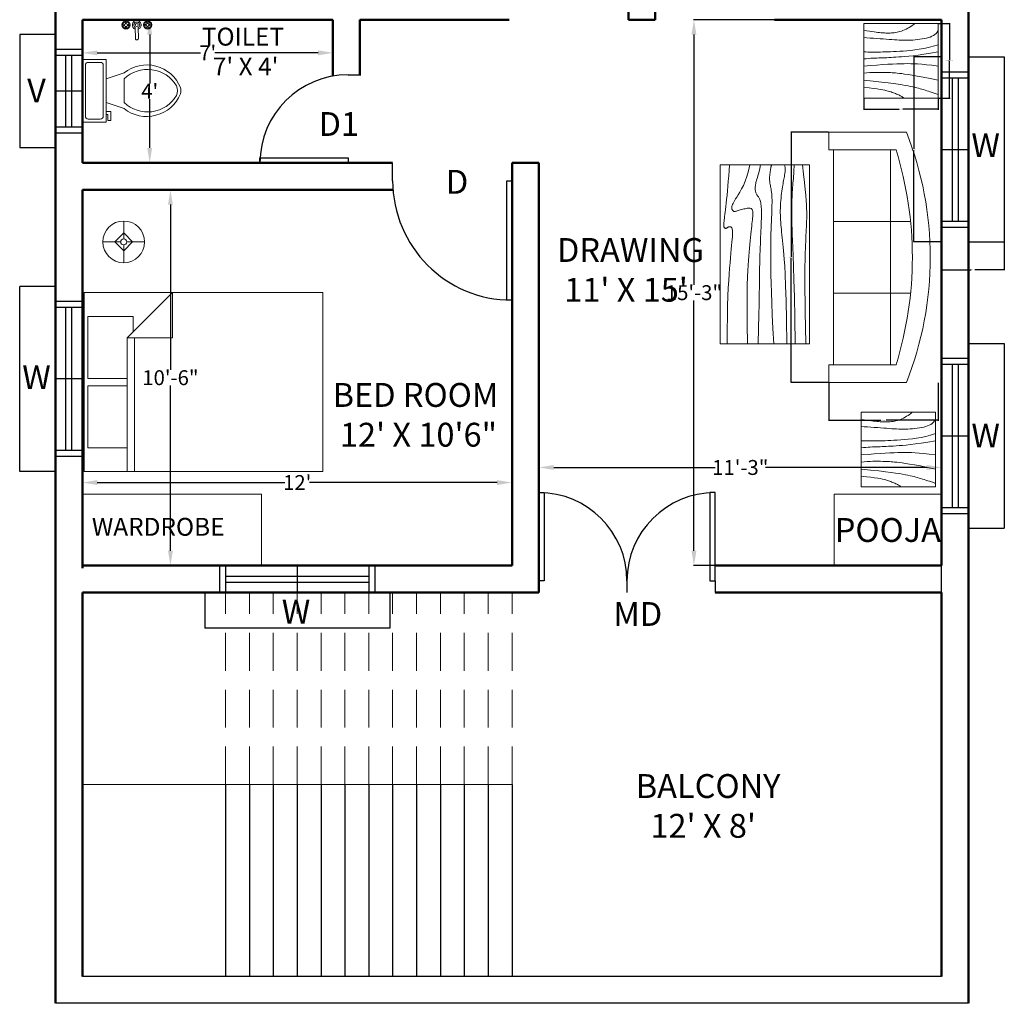
# Model space of a CAD drawing. Units: inches. Extents: x -25 to 789, y -921 to 230.
# Tile 4 of 5: x 437 to 767, y -323 to 6. Entities that reach past the tile are written whole.
import ezdxf

# ---------------------------------------------------------------- set-up
doc = ezdxf.new("R2010")
doc.units = ezdxf.units.IN
doc.header["$MEASUREMENT"] = 0
doc.linetypes.add('DASHED', pattern=[19.05, 12.7, -6.35])
for name, color, linetype, lineweight in [('A-ANNO-DIMS', 2, 'Continuous', 18), ('A-ANNO-TEXT', 7, 'Continuous', 18), ('A-AREA-IDEN', 3, 'Continuous', 18), ('A-DOOR', 4, 'Continuous', 25), ('A-ELEV', 7, 'Continuous', 25), ('A-FLOR-FIXT', 9, 'Continuous', 18), ('A-FLOR-OVHD', 8, 'DASHED', 18), ('A-FLOR-STRS', 3, 'Continuous', 25), ('A-FURN', 8, 'Continuous', 18), ('A-GLAZ', 4, 'Continuous', 25), ('A-WALL', 7, 'Continuous', 50), ('E-LITE-FIXT', 6, 'Continuous', 18)]:
    doc.layers.add(name, color=color, linetype=linetype, lineweight=lineweight)
doc.styles.get("Standard").update_dxf_attribs({"font": 'arial.ttf'})
doc.dimstyles.get("Standard").update_dxf_attribs({"dimtxt": 0.18, "dimasz": 0.18, "dimexe": 0.18, "dimexo": 0.0625, "dimgap": 0.09, "dimtad": 0, "dimtih": 1, "dimtoh": 1, "dimdec": 1, "dimzin": 0, "dimdsep": 46, "dimlunit": 4, "dimtxsty": 'Standard', "dimcen": 0.09, "dimadec": 0, "dimazin": 0, "dimtfac": 1, "dimtdec": 1, "dimtofl": 0, "dimtmove": 0, "dimatfit": 3, "dimfxl": 1, "dimtolj": 1, "dimtzin": 0, "dimarcsym": 0})

# ---------------------------------------------------------------- blocks, each defined once
blk = doc.blocks.new('Toilet - top')
for p, q in [((9.5, -6), (9.5, -2)), ((-10, -8.5), (-8, -8.5)), ((-10, -9.5), (-10, -8.5)), ((-7, -9.5), (-10, -9.5)), ((-8, -8.5), (-8, -8)), ((-7, -8), (-7, -9.5)), ((-4, -8), (-6, -14)), ((4, -8), (6, -14)), ((4, -14), (-4, -14))]:
    blk.add_line(p, q)
blk.add_lwpolyline([(10.5, -8), (10.5, 0), (-10.5, 0), (-10.5, -8)], close=True)
for points in [[(-9.5, -2), (-9.5, -6)], [(8.5, -1), (-8.5, -1)], [(-8.5, -7), (8.5, -7)]]:
    blk.add_lwpolyline(points)
for centre, radius, start, end in [((-8.62, -1.88), 0.884, 81.8699, 188.1301), ((8.62, -1.88), 0.884, 351.8699, 98.1301), ((-8.62, -6.12), 0.884, 171.8699, 278.1301), ((8.62, -6.12), 0.884, 261.8699, 8.1301), ((3.52, -21.58), 12.17, 141.4691, 247.9714), ((4.2, -21.82), 11.33, 136.3677, 238.9468), ((-3.52, -21.58), 12.17, 292.0284, 38.5307), ((-4.2, -21.82), 11.33, 301.053, 43.6321), ((0, -27.88), 4, 245.7318, 294.2682), ((0, -29), 4, 254.8605, 285.1395)]:
    blk.add_arc(centre, radius, start, end)
blk = doc.blocks.new('*U26')
for p, q in [((-40, 0), (-40, 6)), ((0, 0), (0, 6))]:
    blk.add_line(p, q)
blk.add_lwpolyline([(0, 0), (0, -40), (-1.75, -40), (-1.75, 0)], close=True)
blk.add_arc((0, 0), 40, 180, 270)
blk = doc.blocks.new('Faucet - Bathroom top')
for p, q in [((-4.107, 0.125), (-4.375, 0.125)), ((-3.75, 0.4788), (-3.75, 0.75)), ((-3.5, 0.482), (-3.5, 0.75)), ((-3.1461, 0.125), (-2.875, 0.125)), ((3.143, 0.125), (2.875, 0.125)), ((3.5, 0.4788), (3.5, 0.75)), ((3.75, 0.482), (3.75, 0.75)), ((4.1039, 0.125), (4.375, 0.125)), ((-4.1039, -0.125), (-4.375, -0.125)), ((-3.75, -0.4821), (-3.75, -0.75)), ((-3.5, -0.4789), (-3.5, -0.75)), ((-3.143, -0.125), (-2.875, -0.125)), ((-0.5, -0.8639), (-0.5, -4.5)), ((0.5, -4.5), (0.5, -0.8631)), ((3.1461, -0.125), (2.875, -0.125)), ((3.5, -0.4821), (3.5, -0.75)), ((3.75, -0.4789), (3.75, -0.75)), ((4.107, -0.125), (4.375, -0.125))]:
    blk.add_line(p, q)
for centre, radius in [((-3.625, 0), 1.375), ((-4.625, 0), 0.2795), ((-3.625, 0), 0.5), ((-3.625, 1), 0.2795), ((-2.625, 0), 0.2795), ((0, 0), 0.5), ((3.625, 0), 1.375), ((2.625, 0), 0.2795), ((3.625, 0), 0.5), ((3.625, 1), 0.2795), ((4.625, 0), 0.2795), ((-3.625, -1), 0.2795), ((3.625, -1), 0.2795)]:
    blk.add_circle(centre, radius)
for centre, radius, start, end in [((-3.625, 0), 1, 105.2407, 164.2093), ((-3.625, 0), 1, 16.44125, 74.07887), ((0, 0), 1.5, 289.6514, 250.3603), ((0, 0), 1, 300.3431, 239.7554), ((3.625, 0), 1, 106.12, 164.0884), ((3.625, 0), 1, 16.23422, 73.90469), ((-3.625, 0), 1, 196.2342, 253.9047), ((-3.625, 0), 1, 286.12, 344.0884), ((3.625, 0), 1, 196.4413, 254.0789), ((3.625, 0), 1, 285.2407, 344.2093), ((0, -4.5), 0.5, 180, 0)]:
    blk.add_arc(centre, radius, start, end)
blk = doc.blocks.new('*U20')
for p, q in [((-750, 0), (-750, 100)), ((0, 0), (0, 100))]:
    blk.add_line(p, q)
blk.add_lwpolyline([(0, 0), (0, -750), (-43.75, -750), (-43.75, 0)], close=True)
blk.add_arc((0, 0), 750, 180, 270)
blk = doc.blocks.new('Bed - Queen')
for p, q in [((0, -80.00003), (0, 0)), ((0, 0), (59.99999, 0)), ((59.99999, 0), (59.99999, -80.00003)), ((7.99999, -1.2), (28.79998, -1.2)), ((7.99999, -14.4), (7.99999, -1.2)), ((28.79998, -1.2), (28.79998, -14.4)), ((31.19999, -1.2), (51.99999, -1.2)), ((31.19999, -14.4), (31.19999, -1.2)), ((51.99999, -1.2), (51.99999, -16.4)), ((0, -14.4), (44.8, -14.4)), ((59.99999, -29.6), (44.8, -14.4)), ((44.8, -14.4), (44.8, -29.6)), ((51.99999, -16.4), (46.79936, -16.4)), ((44.8, -16.8), (0, -16.8)), ((44.8, -29.6), (59.99999, -29.6)), ((59.99999, -80.00003), (0, -80.00003))]:
    blk.add_line(p, q)
blk = doc.blocks.new('Lamp - Table')
for p, q in [((0, 7), (0, 1)), ((-1, 0), (-7, 0)), ((0, 3), (-3, 0)), ((-3, 0), (0, -3)), ((3, 0), (0, 3)), ((0, -3), (3, 0)), ((1, 0), (7, 0)), ((0, -1), (0, -7))]:
    blk.add_line(p, q)
for radius in [7, 1]:
    blk.add_circle((0, 0), radius)
blk = doc.blocks.new('*U4')
for p, q in [((-750, 0), (-750, -100)), ((0, 0), (0, -100))]:
    blk.add_line(p, q)
blk.add_lwpolyline([(0, 0), (0, 750), (-43.75, 750), (-43.75, 0)], close=True)
blk.add_arc((0, 0), 750, 90, 180)
blk = doc.blocks.new('*U11')
for p, q in [((0, 0), (0, -100)), ((750, 0), (750, -100))]:
    blk.add_line(p, q)
blk.add_lwpolyline([(0, 0), (0, 750), (43.75, 750), (43.75, 0)], close=True)
blk.add_arc((0, 0), 750, 0, 90)
blk = doc.blocks.new('Sofa - Roundback 7 ft.')
for p, q in [((-12.00002, -32.4421), (-12.00003, -6.5971)), ((11.99997, -32.4421), (11.99998, -6.5971)), ((-36.000027, -34), (-36.000027, -11.4696)), ((35.99998, -34), (35.99998, -11.4696)), ((-35.999844, -13.3819), (35.9998, -13.3819)), ((-36.000027, -32.4421), (35.99998, -32.4421))]:
    blk.add_line(p, q)
for points in [[(-36.000027, -34), (-42.000027, -34), (-42.000027, -8)], [(41.99998, -8), (41.99998, -34), (35.99998, -34)]]:
    blk.add_lwpolyline(points)
for centre, radius, start, end in [((0, -114.25), 114.25, 68.43141, 111.5686), ((-0.00001, -127.1968), 121.1968, 72.72033, 107.2797)]:
    blk.add_arc(centre, radius, start, end)
blk = doc.blocks.new('Table - Rectangular Woodgrain 60 x 30 in.')
for p, q in [((0, 0), (0, -30)), ((60, 0), (0, 0)), ((60, -30), (60, 0)), ((0, -30), (60, -30))]:
    blk.add_line(p, q)
for points in [[(0, -2.4), (4.8155, -2.418), (9.0302, -2.4688), (12.709, -2.5477), (15.9167, -2.65), (18.7181, -2.7711), (21.1781, -2.9063), (23.3616, -3.0508), (25.3333, -3.2), (27.1477, -3.3495), (28.8172, -3.4958), (30.3437, -3.636), (31.7291, -3.7667), (32.9756, -3.8849), (34.0849, -3.9875), (35.059, -4.0714), (35.9, -4.1334), (36.6114, -4.1711), (37.2041, -4.1854), (37.6906, -4.1779), (38.0833, -4.15), (38.3948, -4.1034), (38.6375, -4.0396), (38.8239, -3.9602), (38.9666, -3.8667), (39.0764, -3.7608), (39.1573, -3.6448), (39.2116, -3.521), (39.2416, -3.3917), (39.2498, -3.2593), (39.2385, -3.1261), (39.21, -2.9944), (39.1666, -2.8667), (39.111, -2.7447), (39.0468, -2.6281), (38.978, -2.5163), (38.9083, -2.4083), (38.8418, -2.3035), (38.7823, -2.201), (38.7337, -2.1001), (38.7, -2), (38.6844, -1.9003), (38.6875, -1.8021), (38.7094, -1.707), (38.75, -1.6167), (38.8094, -1.5326), (38.8875, -1.4563), (38.9844, -1.3893), (39.1, -1.3333), (39.2351, -1.2896), (39.3937, -1.2583), (39.5804, -1.2396), (39.8, -1.2333), (40.057, -1.2396), (40.3562, -1.2583), (40.7023, -1.2896), (41.1, -1.3333), (41.5547, -1.3895), (42.0755, -1.4573), (42.6721, -1.5361), (43.3542, -1.625), (44.1316, -1.7233), (45.014, -1.8302), (46.0114, -1.9449), (47.1333, -2.0667), (48.3862, -2.1947), (49.7625, -2.3281), (51.2513, -2.4663), (52.8416, -2.6083), (54.5226, -2.7535), (56.2833, -2.9011), (58.1127, -3.0501), (60, -3.2)], [(0, -9.2), (6.5759, -9.0858), (11.9385, -9.0365), (16.2527, -9.0418), (19.6833, -9.0917), (22.3952, -9.1759), (24.5531, -9.2844), (26.322, -9.4069), (27.8666, -9.5333), (29.3241, -9.6553), (30.7203, -9.7719), (32.0532, -9.8837), (33.3208, -9.9917), (34.5213, -10.0965), (35.6526, -10.199), (36.7128, -10.2999), (37.7, -10.4), (38.6129, -10.4996), (39.4531, -10.5969), (40.223, -10.6895), (40.925, -10.775), (41.5613, -10.8512), (42.1344, -10.9156), (42.6465, -10.966), (43.1, -11), (43.4976, -11.0158), (43.8437, -11.0136), (44.143, -10.9942), (44.4, -10.9583), (44.6195, -10.9069), (44.8062, -10.8406), (44.9648, -10.7603), (45.1, -10.6667), (45.2155, -10.5598), (45.3114, -10.4365), (45.3871, -10.2929), (45.4416, -10.125), (45.4743, -9.929), (45.4844, -9.7011), (45.4709, -9.4371), (45.4333, -9.1333), (45.3716, -8.7883), (45.2896, -8.4104), (45.1919, -8.0107), (45.0833, -7.6), (44.9685, -7.1893), (44.8521, -6.7896), (44.7388, -6.4117), (44.6333, -6.0667), (44.54, -5.7628), (44.4614, -5.4979), (44.4001, -5.2675), (44.3583, -5.0667), (44.3384, -4.8909), (44.3427, -4.7354), (44.3736, -4.5956), (44.4333, -4.4667), (44.5236, -4.3453), (44.6427, -4.2333), (44.7884, -4.1339), (44.9583, -4.05), (45.1501, -3.9849), (45.3614, -3.9417), (45.59, -3.9234), (45.8333, -3.9333), (46.0915, -3.9749), (46.3734, -4.0531), (46.6906, -4.1736), (47.0542, -4.3417), (47.4756, -4.5629), (47.9661, -4.8427), (48.5372, -5.1866), (49.2, -5.6), (49.9676, -6.0844), (50.8594, -6.625), (51.8965, -7.2031), (53.1, -7.8), (54.491, -8.3969), (56.0906, -8.975), (57.9199, -9.5156), (60, -10)], [(0, -12.8), (5.1847, -12.9322), (9.6213, -13.0323), (13.3963, -13.1059), (16.5958, -13.1583), (19.3063, -13.1952), (21.614, -13.2219), (23.6054, -13.2439), (25.3666, -13.2667), (26.9728, -13.2947), (28.4531, -13.3281), (29.8256, -13.3663), (31.1083, -13.4083), (32.3191, -13.4535), (33.476, -13.501), (34.597, -13.5501), (35.7, -13.6), (36.7984, -13.6497), (37.8875, -13.6979), (38.9578, -13.743), (40, -13.7833), (41.0047, -13.8174), (41.9625, -13.8438), (42.864, -13.8607), (43.7, -13.8667), (44.4631, -13.8604), (45.1552, -13.8417), (45.7801, -13.8104), (46.3416, -13.7667), (46.8439, -13.7104), (47.2906, -13.6417), (47.6858, -13.5604), (48.0333, -13.4667), (48.3375, -13.3608), (48.6042, -13.2448), (48.8396, -13.121), (49.05, -12.9917), (49.2417, -12.8593), (49.4208, -12.7261), (49.5937, -12.5944), (49.7667, -12.4667), (49.9452, -12.3451), (50.1323, -12.2313), (50.3303, -12.1268), (50.5416, -12.0333), (50.7686, -11.9524), (51.0135, -11.8854), (51.2788, -11.8341), (51.5666, -11.8), (51.8785, -11.7843), (52.2116, -11.7865), (52.562, -11.8059), (52.926, -11.8417), (53.2998, -11.8931), (53.6795, -11.9594), (54.0614, -12.0397), (54.4416, -12.1333), (54.8223, -12.2401), (55.2293, -12.3625), (55.6942, -12.5037), (56.2489, -12.6667), (56.9251, -12.8547), (57.7545, -13.0708), (58.7689, -13.3182), (60, -13.6)], [(0, -18), (5.124, -17.7273), (9.6609, -17.5057), (13.6705, -17.3303), (17.2125, -17.1958), (20.3467, -17.0973), (23.1328, -17.0297), (25.6307, -16.9878), (27.9, -16.9667), (29.9928, -16.9617), (31.9302, -16.9703), (33.7254, -16.9907), (35.3917, -17.0208), (36.9423, -17.0588), (38.3906, -17.1026), (39.7499, -17.1503), (41.0333, -17.2), (42.2519, -17.2496), (43.4073, -17.2969), (44.4986, -17.3395), (45.525, -17.375), (46.4858, -17.4012), (47.3802, -17.4156), (48.2074, -17.416), (48.9667, -17.4), (49.6583, -17.3662), (50.2872, -17.3167), (50.8595, -17.2547), (51.3812, -17.1833), (51.8584, -17.1057), (52.2971, -17.025), (52.7034, -16.9443), (53.0833, -16.8667), (53.443, -16.7951), (53.789, -16.7313), (54.128, -16.6768), (54.4666, -16.6334), (54.8115, -16.6024), (55.1693, -16.5854), (55.5465, -16.5841), (55.95, -16.6), (56.3828, -16.6337), (56.8346, -16.6823), (57.2915, -16.7418), (57.7396, -16.8084), (58.165, -16.878), (58.5539, -16.9469), (58.8924, -17.0111), (59.1666, -17.0667), (59.3679, -17.1107), (59.5078, -17.1438), (59.6032, -17.1675), (59.6708, -17.1833), (59.7275, -17.193), (59.7901, -17.1979), (59.8753, -17.1998), (60, -17.2)], [(0, -22.4), (8.0098, -22.2501), (14.4094, -22.1011), (19.4168, -21.9535), (23.25, -21.8083), (26.1269, -21.6663), (28.2656, -21.5281), (29.884, -21.3947), (31.2, -21.2667), (32.3967, -21.1448), (33.5172, -21.0292), (34.5697, -20.9198), (35.5625, -20.8167), (36.5037, -20.7198), (37.4015, -20.6292), (38.2642, -20.5448), (39.1, -20.4667), (39.9164, -20.3951), (40.7187, -20.3313), (41.5117, -20.2768), (42.3, -20.2333), (43.0883, -20.2024), (43.8812, -20.1854), (44.6836, -20.1841), (45.5, -20.2), (46.3328, -20.234), (47.1747, -20.2844), (48.0163, -20.3488), (48.8479, -20.425), (49.66, -20.5106), (50.4429, -20.6031), (51.1872, -20.7004), (51.8833, -20.8), (52.5246, -20.8999), (53.1166, -20.9995), (53.6681, -21.0983), (54.1875, -21.1958), (54.6834, -21.2919), (55.1646, -21.3859), (55.6394, -21.4777), (56.1167, -21.5667), (56.6028, -21.6515), (57.0961, -21.7266), (57.5929, -21.7852), (58.0896, -21.8208), (58.5823, -21.8268), (59.0674, -21.7964), (59.5412, -21.723), (60, -21.6)], [(0, -25.2), (8.6355, -25.0504), (15.7026, -24.9031), (21.4049, -24.7606), (25.9458, -24.625), (29.529, -24.4988), (32.3578, -24.3844), (34.6359, -24.284), (36.5667, -24.2), (38.3213, -24.1341), (39.9417, -24.0854), (41.437, -24.0523), (42.8167, -24.0333), (44.0901, -24.0268), (45.2667, -24.0313), (46.3557, -24.0451), (47.3667, -24.0667), (48.309, -24.0947), (49.1928, -24.1287), (50.0284, -24.168), (50.826, -24.2125), (51.5959, -24.2617), (52.3483, -24.3151), (53.0935, -24.3725), (53.8417, -24.4334), (54.6009, -24.497), (55.3699, -24.561), (56.1454, -24.6226), (56.9239, -24.6792), (57.7021, -24.7279), (58.4764, -24.7662), (59.2435, -24.7911), (60, -24.8)], [(0, -28.8), (5.6867, -28.6681), (10.45, -28.5698), (14.407, -28.5012), (17.675, -28.4584), (20.3711, -28.4374), (22.6125, -28.4344), (24.5164, -28.4455), (26.2, -28.4667), (27.762, -28.4947), (29.2276, -28.5281), (30.6033, -28.5663), (31.8958, -28.6084), (33.1118, -28.6535), (34.2578, -28.7011), (35.3405, -28.7501), (36.3666, -28.8), (37.3443, -28.8497), (38.288, -28.8974), (39.2137, -28.9412), (40.1375, -28.9792), (41.0753, -29.0093), (42.0432, -29.0297), (43.0572, -29.0384), (44.1333, -29.0333), (45.2936, -29.0114), (46.5843, -28.9641), (48.0579, -28.8816), (49.7666, -28.7542), (51.7629, -28.5721), (54.0989, -28.3255), (56.8272, -28.0048), (60, -27.6)]]:
    blk.add_lwpolyline(points)
blk = doc.blocks.new('Table - Square Woodgrain 42 x 42 in.')
blk.add_line((0, -42), (42, -42))
for points in [[(0, -4), (1.704, -4.2172), (3.2358, -4.4188), (4.615, -4.604), (5.8615, -4.7721), (6.9951, -4.9224), (8.0357, -5.0541), (9.0031, -5.1667), (9.9171, -5.2594), (10.7951, -5.3316), (11.6445, -5.3836), (12.4702, -5.4157), (13.277, -5.4283), (14.0698, -5.4217), (14.8535, -5.3964), (15.6331, -5.3526), (16.4133, -5.2908), (17.1986, -5.2103), (17.9913, -5.1062), (18.793, -4.9727), (19.6056, -4.8038), (20.4307, -4.5937), (21.2701, -4.3365), (22.1256, -4.0262), (22.9989, -3.6571), (23.888, -3.2272), (24.7756, -2.7516), (25.6408, -2.2491), (26.4624, -1.7387), (27.2195, -1.2395), (27.891, -0.7703), (28.456, -0.3501), (28.8934, 0.002)], [(0, -42), (0, 0), (42, 0), (42, -42)], [(0, -8), (1.8203, -8.1001), (3.6741, -8.2149), (5.5411, -8.3408), (7.4011, -8.4741), (9.2339, -8.6112), (11.0193, -8.7484), (12.7371, -8.8821), (14.3671, -9.0086), (15.8954, -9.1246), (17.3337, -9.2278), (18.6997, -9.3159), (20.0116, -9.387), (21.2871, -9.4389), (22.5442, -9.4696), (23.8008, -9.477), (25.0749, -9.459), (26.3791, -9.4137), (27.7049, -9.3403), (29.0383, -9.2382), (30.3655, -9.1068), (31.6728, -8.9455), (32.9461, -8.7535), (34.1717, -8.5304), (35.3358, -8.2756), (36.4268, -7.9863), (37.443, -7.6521), (38.3849, -7.2603), (39.253, -6.7986), (40.048, -6.2542), (40.7705, -5.6147), (41.421, -4.8674), (42, -4)], [(42, -12), (39.1784, -12.8621), (36.4519, -13.5654), (33.8246, -14.1294), (31.3004, -14.5731), (28.8832, -14.9161), (26.577, -15.1775), (24.3858, -15.3768), (22.3136, -15.5332), (20.3622, -15.6632), (18.5254, -15.7718), (16.7947, -15.8612), (15.1618, -15.9338), (13.6183, -15.9916), (12.1558, -16.0369), (10.7659, -16.0718), (9.4403, -16.0987), (8.1703, -16.1191), (6.9461, -16.1325), (5.7577, -16.1377), (4.595, -16.1335), (3.4479, -16.1188), (2.3064, -16.0924), (1.1604, -16.0532), (0, -16)], [(42, -16), (37.6529, -16.7365), (33.8802, -17.329), (30.6179, -17.7961), (27.8015, -18.1561), (25.3668, -18.4275), (23.2497, -18.6288), (21.3859, -18.7785), (19.7111, -18.8949), (18.1693, -18.9939), (16.7375, -19.0795), (15.401, -19.1534), (14.1449, -19.217), (12.9544, -19.2717), (11.8148, -19.3191), (10.7113, -19.3606), (9.6291, -19.3976), (8.5534, -19.4323), (7.47, -19.4689), (6.3643, -19.5122), (5.222, -19.5672), (4.0288, -19.6386), (2.7703, -19.7313), (1.4321, -19.8501), (0, -20)], [(0, -24), (3.9243, -23.6805), (7.4766, -23.4138), (10.6891, -23.1954), (13.5943, -23.0205), (16.2247, -22.8847), (18.6125, -22.7832), (20.7903, -22.7116), (22.7903, -22.6651), (24.6563, -22.642), (26.4764, -22.6507), (28.35, -22.7024), (30.3766, -22.8084), (32.6555, -22.98), (35.2861, -23.2283), (38.3678, -23.5645), (42, -24)], [(42, -32), (37.392, -31.017), (33.4585, -30.2231), (30.1291, -29.5949), (27.3334, -29.109), (25.0009, -28.742), (23.0612, -28.4707), (21.4439, -28.2716), (20.0786, -28.1215), (18.8998, -28.0002), (17.8609, -27.9014), (16.9206, -27.8219), (16.0371, -27.7588), (15.1691, -27.709), (14.2748, -27.6693), (13.3128, -27.6368), (12.2415, -27.6083), (11.0295, -27.5824), (9.6867, -27.5643), (8.233, -27.5608), (6.6884, -27.5787), (5.0728, -27.6248), (3.4062, -27.7058), (1.7086, -27.8286), (0, -28)], [(0, -32), (5.4026, -32.5358), (9.9494, -33.019), (13.7424, -33.4553), (16.8834, -33.8505), (19.4743, -34.2106), (21.6171, -34.5413), (23.4136, -34.8486), (24.9657, -35.1382), (26.3614, -35.4156), (27.6332, -35.6841), (28.7995, -35.9467), (29.8788, -36.2064), (30.8897, -36.4661), (31.8507, -36.7288), (32.7802, -36.9973), (33.6968, -37.2747), (34.6175, -37.5635), (35.5531, -37.8651), (36.5128, -38.1805), (37.506, -38.5108), (38.5421, -38.8568), (39.6302, -39.2197), (40.7797, -39.6004), (42, -40)], [(0, -36), (3.0098, -36.2857), (5.5354, -36.5643), (7.6368, -36.8359), (9.374, -37.1009), (10.807, -37.3597), (11.9957, -37.6126), (13.0002, -37.8599), (13.8804, -38.102), (14.6874, -38.3393), (15.4365, -38.5729), (16.1338, -38.8041), (16.7858, -39.0341), (17.3987, -39.264), (17.9787, -39.4952), (18.5322, -39.7288), (19.0655, -39.9662), (19.5832, -40.2081), (20.0842, -40.4544), (20.5657, -40.7046), (21.0249, -40.9581), (21.459, -41.2144), (21.8653, -41.4731), (22.2409, -41.7335), (22.5831, -41.9951)]]:
    blk.add_lwpolyline(points)
blk = doc.blocks.new('*D59')
at = {"layer": 'A-ANNO-DIMS', "color": 0, "lineweight": -2, "transparency": 16777216}
for p, q in [((458.24, -176.64), (458.24, -148.68)), ((463.24, -148.86), (526.14, -148.86)), ((597.24, -148.86), (534.33, -148.86)), ((602.24, -176.64), (602.24, -148.68))]:
    blk.add_line(p, q, dxfattribs=at)
at = {"layer": 'A-ANNO-DIMS', "color": 0, "transparency": 16777216}
for points in [[(463.24, -148.02), (463.24, -149.69), (458.24, -148.86)], [(597.24, -148.02), (597.24, -149.69), (602.24, -148.86)]]:
    blk.add_solid(points, dxfattribs=at)
at = {"layer": 'Defpoints', "color": 0, "transparency": 16777216}
for p in [(602.24, -148.86), (458.24, -176.7), (602.24, -176.7)]:
    blk.add_point(p, dxfattribs=at)
at = {"layer": 'A-ANNO-DIMS', "color": 0, "transparency": 16777216, "insert": (530.24, -148.86), "char_height": 5, "attachment_point": 5}
blk.add_mtext("\\A1;12'", dxfattribs=at)
blk = doc.blocks.new('*D60')
at = {"layer": 'A-ANNO-DIMS', "color": 0, "lineweight": -2, "transparency": 16777216}
for p, q in [((458.3, -50.7), (487.93, -50.7)), ((487.75, -55.7), (487.75, -111.06)), ((487.75, -171.7), (487.75, -116.35)), ((458.3, -176.7), (487.93, -176.7))]:
    blk.add_line(p, q, dxfattribs=at)
at = {"layer": 'A-ANNO-DIMS', "color": 0, "transparency": 16777216}
for points in [[(486.92, -55.7), (488.59, -55.7), (487.75, -50.7)], [(486.92, -171.7), (488.59, -171.7), (487.75, -176.7)]]:
    blk.add_solid(points, dxfattribs=at)
at = {"layer": 'Defpoints', "color": 0, "transparency": 16777216}
for p in [(458.24, -50.7), (487.75, -50.7), (458.24, -176.7)]:
    blk.add_point(p, dxfattribs=at)
at = {"layer": 'A-ANNO-DIMS', "color": 0, "transparency": 16777216, "insert": (487.75, -113.7), "char_height": 5, "attachment_point": 5}
blk.add_mtext('\\A1;10\'-6"', dxfattribs=at)
blk = doc.blocks.new('*D61')
at = {"layer": 'A-ANNO-DIMS', "color": 0, "lineweight": -2, "transparency": 16777216}
for p, q in [((458.3, 6.3), (480.99, 6.3)), ((480.81, 1.3), (480.81, -15.11)), ((480.81, -36.7), (480.81, -20.29)), ((458.3, -41.7), (480.99, -41.7))]:
    blk.add_line(p, q, dxfattribs=at)
at = {"layer": 'A-ANNO-DIMS', "color": 0, "transparency": 16777216}
for points in [[(479.97, 1.3), (481.64, 1.3), (480.81, 6.3)], [(479.97, -36.7), (481.64, -36.7), (480.81, -41.7)]]:
    blk.add_solid(points, dxfattribs=at)
at = {"layer": 'Defpoints', "color": 0, "transparency": 16777216}
for p in [(458.24, 6.3), (480.81, 6.3), (458.24, -41.7)]:
    blk.add_point(p, dxfattribs=at)
at = {"layer": 'A-ANNO-DIMS', "color": 0, "transparency": 16777216, "insert": (480.81, -17.7), "char_height": 5, "attachment_point": 5}
blk.add_mtext("\\A1;4'", dxfattribs=at)
blk = doc.blocks.new('*D62')
at = {"layer": 'A-ANNO-DIMS', "color": 0, "lineweight": -2, "transparency": 16777216}
for p, q in [((458.24, 6.23), (458.24, -5)), ((542.24, 6.23), (542.24, -5)), ((463.24, -4.82), (497.87, -4.82)), ((537.24, -4.82), (502.61, -4.82))]:
    blk.add_line(p, q, dxfattribs=at)
at = {"layer": 'A-ANNO-DIMS', "color": 0, "transparency": 16777216}
for points in [[(463.24, -3.99), (463.24, -5.65), (458.24, -4.82)], [(537.24, -3.99), (537.24, -5.65), (542.24, -4.82)]]:
    blk.add_solid(points, dxfattribs=at)
at = {"layer": 'Defpoints', "color": 0, "transparency": 16777216}
for p in [(458.24, 6.3), (542.24, 6.3), (542.24, -4.82)]:
    blk.add_point(p, dxfattribs=at)
at = {"layer": 'A-ANNO-DIMS', "color": 0, "transparency": 16777216, "insert": (500.24, -4.82), "char_height": 5, "attachment_point": 5}
blk.add_mtext("\\A1;7'", dxfattribs=at)
blk = doc.blocks.new('*D71')
at = {"layer": 'A-ANNO-DIMS', "color": 0, "lineweight": -2, "transparency": 16777216}
for p, q in [((611.24, -185.64), (611.24, -143.62)), ((616.24, -143.8), (670.29, -143.8)), ((741.24, -143.8), (687.18, -143.8)), ((746.24, -185.64), (746.24, -143.62))]:
    blk.add_line(p, q, dxfattribs=at)
at = {"layer": 'A-ANNO-DIMS', "color": 0, "transparency": 16777216}
for points in [[(616.24, -142.97), (616.24, -144.64), (611.24, -143.8)], [(741.24, -142.97), (741.24, -144.64), (746.24, -143.8)]]:
    blk.add_solid(points, dxfattribs=at)
at = {"layer": 'Defpoints', "color": 0, "transparency": 16777216}
for p in [(746.24, -143.8), (611.24, -185.7), (746.24, -185.7)]:
    blk.add_point(p, dxfattribs=at)
at = {"layer": 'A-ANNO-DIMS', "color": 0, "transparency": 16777216, "insert": (678.74, -143.8), "char_height": 5, "attachment_point": 5}
blk.add_mtext('\\A1;11\'-3"', dxfattribs=at)
blk = doc.blocks.new('*D72')
at = {"layer": 'A-ANNO-DIMS', "color": 0, "lineweight": -2, "transparency": 16777216}
for p, q in [((690.17, 6.3), (663.04, 6.3)), ((663.22, 1.3), (663.22, -82.56)), ((663.22, -171.7), (663.22, -87.85)), ((670.23, -176.7), (663.04, -176.7))]:
    blk.add_line(p, q, dxfattribs=at)
at = {"layer": 'A-ANNO-DIMS', "color": 0, "transparency": 16777216}
for points in [[(662.38, 1.3), (664.05, 1.3), (663.22, 6.3)], [(662.38, -171.7), (664.05, -171.7), (663.22, -176.7)]]:
    blk.add_solid(points, dxfattribs=at)
at = {"layer": 'Defpoints', "color": 0, "transparency": 16777216}
for p in [(663.22, 6.3), (690.24, 6.3), (670.29, -176.7)]:
    blk.add_point(p, dxfattribs=at)
at = {"layer": 'A-ANNO-DIMS', "color": 0, "transparency": 16777216, "insert": (663.22, -85.2), "char_height": 5, "attachment_point": 5}
blk.add_mtext('\\A1;15\'-3"', dxfattribs=at)
blk = doc.blocks.new('WIN-W-SUNSHADE')
at = {"ltscale": 2}
for p, q in [((0, 9), (0, 21)), ((0, 21), (62, 21)), ((62, 9), (62, 21)), ((5, 9), (0, 9)), ((57, 9), (62, 9))]:
    blk.add_line(p, q, dxfattribs=at)
for p, q in [((5, 0), (5, 9)), ((57, 0), (57, 9))]:
    blk.add_line(p, q)
blk = doc.blocks.new('WIN-V-SUNSHADE')
for p, q in [((0, 9), (0, 21)), ((38, 21), (0, 21)), ((38, 9), (38, 21)), ((5, 9), (0, 9)), ((5, 0), (5, 9)), ((33, 0), (33, 9)), ((33, 9), (38, 9))]:
    blk.add_line(p, q)
blk = doc.blocks.new('*D81')
at = {"layer": 'A-ANNO-DIMS', "color": 0, "lineweight": -2, "transparency": 16777216}
for p, q in [((746.17, -6.2), (736.76, -6.2)), ((736.94, -6.38), (736.94, -37.02)), ((736.94, -68.02), (736.94, -37.39)), ((746.17, -68.2), (736.76, -68.2))]:
    blk.add_line(p, q, dxfattribs=at)
at = {"layer": 'A-ANNO-DIMS', "color": 0, "transparency": 16777216}
for points in [[(736.91, -6.38), (736.97, -6.38), (736.94, -6.2)], [(736.91, -68.02), (736.97, -68.02), (736.94, -68.2)]]:
    blk.add_solid(points, dxfattribs=at)
at = {"layer": 'Defpoints', "color": 0, "transparency": 16777216}
for p in [(746.24, -6.2), (736.94, -68.2), (746.24, -68.2)]:
    blk.add_point(p, dxfattribs=at)
at = {"layer": 'A-ANNO-DIMS', "color": 0, "transparency": 16777216, "insert": (736.94, -37.2), "char_height": 0.18, "attachment_point": 5}
blk.add_mtext('\\A1;WINDOW W 5\'-2" TYP.', dxfattribs=at)
blk = doc.blocks.new('*D82')
at = {"layer": 'A-ANNO-DIMS', "color": 0, "lineweight": -2, "transparency": 16777216}
for p, q in [((746.24, -68.27), (746.24, -77.68)), ((767.24, -68.27), (767.24, -77.68)), ((746.42, -77.5), (756.11, -77.5)), ((767.06, -77.5), (757.37, -77.5))]:
    blk.add_line(p, q, dxfattribs=at)
at = {"layer": 'A-ANNO-DIMS', "color": 0, "transparency": 16777216}
for points in [[(746.42, -77.47), (746.42, -77.53), (746.24, -77.5)], [(767.06, -77.47), (767.06, -77.53), (767.24, -77.5)]]:
    blk.add_solid(points, dxfattribs=at)
at = {"layer": 'Defpoints', "color": 0, "transparency": 16777216}
for p in [(746.24, -68.2), (767.24, -68.2), (767.24, -77.5)]:
    blk.add_point(p, dxfattribs=at)
at = {"layer": 'A-ANNO-DIMS', "color": 0, "transparency": 16777216, "insert": (756.74, -77.5), "char_height": 0.18, "attachment_point": 5}
blk.add_mtext('\\A1;1\'-9" TYP.', dxfattribs=at)
blk = doc.blocks.new('*D93')
at = {"layer": 'A-ANNO-DIMS', "color": 0, "lineweight": -2, "transparency": 16777216}
for p, q in [((708.35, -31.37), (695.64, -31.37)), ((695.82, -31.55), (695.82, -73.18)), ((695.82, -115.19), (695.82, -73.55)), ((708.35, -115.37), (695.64, -115.37))]:
    blk.add_line(p, q, dxfattribs=at)
at = {"layer": 'A-ANNO-DIMS', "color": 0, "transparency": 16777216}
for points in [[(695.79, -31.55), (695.85, -31.55), (695.82, -31.37)], [(695.79, -115.19), (695.85, -115.19), (695.82, -115.37)]]:
    blk.add_solid(points, dxfattribs=at)
at = {"layer": 'Defpoints', "color": 0, "transparency": 16777216}
for p in [(708.42, -31.37), (695.82, -115.37), (708.42, -115.37)]:
    blk.add_point(p, dxfattribs=at)
at = {"layer": 'A-ANNO-DIMS', "color": 0, "transparency": 16777216, "insert": (695.82, -73.37), "char_height": 0.18, "attachment_point": 5}
blk.add_mtext('\\A1;SOFA 7\'-0" TYP.', dxfattribs=at)
blk = doc.blocks.new('*D94')
at = {"layer": 'A-ANNO-DIMS', "color": 0, "lineweight": -2, "transparency": 16777216}
for p, q in [((708.42, -115.43), (708.42, -128.15)), ((745.08, -115.43), (745.08, -128.15)), ((708.6, -127.97), (725.9, -127.97)), ((744.9, -127.97), (727.6, -127.97))]:
    blk.add_line(p, q, dxfattribs=at)
at = {"layer": 'A-ANNO-DIMS', "color": 0, "transparency": 16777216}
for points in [[(708.6, -127.94), (708.6, -128), (708.42, -127.97)], [(744.9, -127.94), (744.9, -128), (745.08, -127.97)]]:
    blk.add_solid(points, dxfattribs=at)
at = {"layer": 'Defpoints', "color": 0, "transparency": 16777216}
for p in [(708.42, -115.37), (745.08, -115.37), (745.08, -127.97)]:
    blk.add_point(p, dxfattribs=at)
at = {"layer": 'A-ANNO-DIMS', "color": 0, "transparency": 16777216, "insert": (726.75, -127.97), "char_height": 0.18, "attachment_point": 5}
blk.add_mtext('\\A1;3\'-0 1/2" TYP.', dxfattribs=at)
blk = doc.blocks.new('*D95')
at = {"layer": 'A-ANNO-DIMS', "color": 0, "lineweight": -2, "transparency": 16777216}
for p, q in [((745.17, 5.04), (749.04, 5.04)), ((748.86, 4.86), (748.86, -7.28)), ((748.86, -19.79), (748.86, -7.65)), ((745.17, -19.97), (749.04, -19.97))]:
    blk.add_line(p, q, dxfattribs=at)
at = {"layer": 'A-ANNO-DIMS', "color": 0, "transparency": 16777216}
for points in [[(748.83, 4.86), (748.89, 4.86), (748.86, 5.04)], [(748.83, -19.79), (748.89, -19.79), (748.86, -19.97)]]:
    blk.add_solid(points, dxfattribs=at)
at = {"layer": 'Defpoints', "color": 0, "transparency": 16777216}
for p in [(745.11, 5.04), (748.86, 5.04), (745.11, -19.97)]:
    blk.add_point(p, dxfattribs=at)
at = {"layer": 'A-ANNO-DIMS', "color": 0, "transparency": 16777216, "insert": (748.86, -7.46), "char_height": 0.18, "attachment_point": 5}
blk.add_mtext('\\A1;SIDE TABLE 2\'-1" TYP.', dxfattribs=at)
blk = doc.blocks.new('*D96')
at = {"layer": 'A-ANNO-DIMS', "color": 0, "lineweight": -2, "transparency": 16777216}
for p, q in [((720.1, -20.03), (720.1, -23.9)), ((745.11, -20.03), (745.11, -23.9)), ((720.28, -23.72), (731.96, -23.72)), ((744.93, -23.72), (733.24, -23.72))]:
    blk.add_line(p, q, dxfattribs=at)
at = {"layer": 'A-ANNO-DIMS', "color": 0, "transparency": 16777216}
for points in [[(720.28, -23.69), (720.28, -23.75), (720.1, -23.72)], [(744.93, -23.69), (744.93, -23.75), (745.11, -23.72)]]:
    blk.add_solid(points, dxfattribs=at)
at = {"layer": 'Defpoints', "color": 0, "transparency": 16777216}
for p in [(720.1, -19.97), (745.11, -19.97), (745.11, -23.72)]:
    blk.add_point(p, dxfattribs=at)
at = {"layer": 'A-ANNO-DIMS', "color": 0, "transparency": 16777216, "insert": (732.6, -23.72), "char_height": 0.18, "attachment_point": 5}
blk.add_mtext('\\A1;2\'-1" TYP.', dxfattribs=at)

msp = doc.modelspace()

# ---------------------------------------------------------------- linework, layer by layer
at = {"layer": 'A-ELEV'}
for p, q in [((746.24, -314.42), (458.24, -314.42)), ((755.24, -323.42), (449.24, -323.42))]:
    msp.add_line(p, q, dxfattribs=at)
at = {"layer": 'A-FLOR-OVHD'}
for p, q in [((506.24, -250.06), (506.24, -185.7)), ((514.24, -250.06), (514.24, -185.7)), ((522.24, -250.06), (522.24, -185.7)), ((530.24, -250.06), (530.24, -185.7)), ((538.24, -250.06), (538.24, -185.7)), ((546.24, -250.06), (546.24, -185.7)), ((554.24, -250.06), (554.24, -185.7)), ((562.24, -250.06), (562.24, -185.7)), ((570.24, -250.06), (570.24, -185.7)), ((578.24, -250.06), (578.24, -185.7)), ((586.24, -250.06), (586.24, -185.7)), ((594.24, -250.06), (594.24, -185.7)), ((602.24, -250.06), (602.24, -185.7))]:
    msp.add_line(p, q, dxfattribs=at)
at = {"layer": 'A-FLOR-STRS'}
for p, q in [((506.24, -250.06), (506.24, -314.42)), ((514.24, -250.06), (514.24, -314.42)), ((522.24, -250.06), (522.24, -314.42)), ((530.24, -250.06), (530.24, -314.42)), ((538.24, -250.06), (538.24, -314.42)), ((546.24, -250.06), (546.24, -314.42)), ((554.24, -250.06), (554.24, -314.42)), ((562.24, -250.06), (562.24, -314.42)), ((570.24, -250.06), (570.24, -314.42)), ((578.24, -250.06), (578.24, -314.42)), ((586.24, -250.06), (586.24, -314.42)), ((594.24, -250.06), (594.24, -314.42)), ((602.24, -250.06), (602.24, -314.42))]:
    msp.add_line(p, q, dxfattribs=at)
at = {"layer": 'A-FURN'}
for p, q in [((458.24, -50.7), (542.24, -50.7)), ((458.24, -176.7), (458.24, -152.7)), ((458.24, -152.7), (518.24, -152.7)), ((518.24, -152.7), (518.24, -176.7)), ((710.24, -176.7), (710.24, -152.7)), ((710.24, -152.7), (746.24, -152.7)), ((746.24, -176.7), (710.24, -176.7)), ((458.24, -250.06), (602.24, -250.06))]:
    msp.add_line(p, q, dxfattribs=at)
at = {"layer": 'A-GLAZ'}
for p, q in [((458.24, -5.7), (449.24, -5.7)), ((452.74, -29.7), (452.74, -5.7)), ((454.74, -29.7), (454.74, -5.7)), ((746.24, -13.2), (755.24, -13.2)), ((749.74, -13.2), (749.74, -61.2)), ((751.74, -13.2), (751.74, -61.2)), ((458.24, -17.7), (449.24, -17.7)), ((458.24, -29.7), (449.24, -29.7)), ((746.24, -37.2), (755.24, -37.2)), ((746.24, -61.2), (755.24, -61.2)), ((458.24, -90.13), (449.24, -90.13)), ((452.74, -138.13), (452.74, -90.13)), ((454.74, -138.13), (454.74, -90.13)), ((746.24, -109.2), (755.24, -109.2)), ((749.74, -109.2), (749.74, -157.2)), ((751.74, -109.2), (751.74, -157.2)), ((458.24, -114.13), (449.24, -114.13)), ((746.24, -133.2), (755.24, -133.2)), ((458.24, -138.13), (449.24, -138.13)), ((746.24, -157.2), (755.24, -157.2)), ((506.24, -176.7), (506.24, -185.7)), ((530.24, -176.7), (530.24, -185.7)), ((554.24, -176.7), (554.24, -185.7)), ((506.24, -180.2), (554.24, -180.2)), ((506.24, -182.2), (554.24, -182.2))]:
    msp.add_line(p, q, dxfattribs=at)
at = {"layer": 'A-WALL'}
for p, q in [((449.24, 6.3), (449.24, 198.3)), ((755.24, 198.3), (755.24, 6.3)), ((641.24, 160.03), (641.24, 6.3)), ((650.24, 132.3), (650.24, 6.3)), ((755.24, 15.3), (755.24, -323.42)), ((449.24, 6.3), (449.24, -50.7)), ((458.24, 6.3), (458.24, -41.7)), ((542.24, 6.3), (458.24, 6.3)), ((542.24, -12.61), (542.24, 6.3)), ((551.24, -12.44), (551.24, 6.3)), ((601.24, 6.3), (551.24, 6.3)), ((650.24, 6.3), (641.24, 6.3)), ((746.24, 6.3), (690.24, 6.3)), ((746.24, 6.3), (746.24, -176.7)), ((458.24, -41.7), (562.24, -41.7)), ((602.24, -176.7), (602.24, -41.7)), ((602.24, -41.7), (611.24, -41.7)), ((611.24, -185.7), (611.24, -41.7)), ((449.24, -50.7), (449.24, -323.42)), ((458.24, -50.7), (458.24, -177.55)), ((562.35, -50.7), (458.24, -50.7)), ((458.24, -176.7), (602.24, -176.7)), ((670.29, -176.7), (746.24, -176.7)), ((458.24, -185.7), (611.24, -185.7)), ((458.24, -185.7), (458.24, -314.42)), ((670.29, -185.7), (746.24, -185.7)), ((746.24, -185.7), (746.24, -314.42))]:
    msp.add_line(p, q, dxfattribs=at)

# ---------------------------------------------------------------- block references
at = {"layer": 'A-DOOR', "xscale": 0.0393700787401575, "yscale": 0.0393700787401575, "zscale": 0.0393700787401575, "rotation": 270}
msp.add_blockref('*U20', (547.3, -41.7), dxfattribs=at)
at = {"layer": 'A-DOOR'}
msp.add_blockref('*U26', (602.24, -47.7), dxfattribs=at)
at = {"layer": 'A-DOOR', "xscale": 0.0393700787401575, "yscale": 0.0393700787401575, "zscale": 0.0393700787401575}
for name, p in [('*U11', (611.24, -181.77)), ('*U4', (670.29, -181.77))]:
    msp.add_blockref(name, p, dxfattribs=at)
at = {"layer": 'A-FLOR-FIXT'}
for name, p, rotation in [('Faucet - Bathroom top', (476.48, 4.52), 0.4207759657041173), ('Toilet - top', (458.24, -17.51), 90)]:
    msp.add_blockref(name, p, dxfattribs=dict(at, rotation=rotation))
at = {"layer": 'A-FURN', "xscale": 0.595437284280929, "yscale": 0.595437284280929, "zscale": 0.595437284280929}
for p in [(720.1, 5.04), (719.22, -125.31)]:
    msp.add_blockref('Table - Square Woodgrain 42 x 42 in.', p, dxfattribs=at)
at = {"layer": 'A-FURN'}
for name, p, rotation in [('Sofa - Roundback 7 ft.', (742.42, -73.37), 270), ('Table - Rectangular Woodgrain 60 x 30 in.', (671.97, -102.34), 90), ('Bed - Queen', (458.89, -145.19), 90)]:
    msp.add_blockref(name, p, dxfattribs=dict(at, rotation=rotation))
at = {"layer": 'A-GLAZ'}
for name, p, rotation in [('WIN-V-SUNSHADE', (458.24, -36.7), 89.99999999999966), ('WIN-W-SUNSHADE', (746.24, -6.2), 270.0000000000002), ('WIN-W-SUNSHADE', (458.24, -145.13), 90.00000000000026), ('WIN-W-SUNSHADE', (746.24, -102.2), 270.0000000000002), ('WIN-W-SUNSHADE', (561.24, -176.7), 180)]:
    msp.add_blockref(name, p, dxfattribs=dict(at, rotation=rotation))
at = {"layer": 'E-LITE-FIXT'}
msp.add_blockref('Lamp - Table', (472.09, -68.19), dxfattribs=at)

# ---------------------------------------------------------------- texts
at = {"layer": 'A-ANNO-TEXT'}
for s, p in [('V', (439.72, -21.42)), ('D1', (537.4, -32.67)), ('W', (756.19, -39.78)), ('D', (580.07, -52.05)), ('W', (438.08, -117.54)), ('W', (756.19, -137.08)), ('W', (525.06, -196.11)), ('MD', (636.21, -196.92))]:
    msp.add_text(s, height=8, dxfattribs=at).set_placement(p)
at = {"layer": 'A-AREA-IDEN', "attachment_point": 1}
for s, insert, char_height in [(" TOILET\\P   7' X 4'", (496.46, 3.61), 6), ("DRAWING\\P 11' X 15'", (617.3, -66.91), 8), ('BED ROOM\\P 12\' X 10\'6"', (542.11, -115.49), 8), ('WARDROBE', (461.42, -160.69), 6), ('POOJA', (710.42, -160.76), 8), ("BALCONY\\P  12' X 8'", (643.73, -246.59), 8)]:
    msp.add_mtext_dynamic_manual_height_columns(s, width=99.8363, gutter_width=1, heights=[0], dxfattribs=dict(at, insert=insert, char_height=char_height))

# ---------------------------------------------------------------- dimensions: what is measured, and where the dimension line sits
at = {"layer": 'A-ANNO-DIMS'}
for base, p1, p2, picture, middle in [((480.81, 6.3), (458.24, -41.7), (458.24, 6.3), '*D61', (480.81, -17.7)), ((663.22, 6.3), (670.29, -176.7), (690.24, 6.3), '*D72', (663.22, -85.2)), ((487.75, -50.7), (458.24, -176.7), (458.24, -50.7), '*D60', (487.75, -113.7))]:
    dim = msp.add_linear_dim(base=base, p1=p1, p2=p2, angle=90, dimstyle='Standard', override={"dimtxt": 5, "dimasz": 5, "dimclrd": 0, "dimclre": 0, "dimclrt": 0}, dxfattribs=at)
    dim.commit()
    dim.dimension.update_dxf_attribs({"geometry": picture, "text_midpoint": middle})
for base, p1, p2, picture, middle in [((542.24, -4.82), (458.24, 6.3), (542.24, 6.3), '*D62', (500.24, -4.82)), ((746.24, -143.8), (611.24, -185.7), (746.24, -185.7), '*D71', (678.74, -143.8)), ((602.24, -148.86), (458.24, -176.7), (602.24, -176.7), '*D59', (530.24, -148.86))]:
    dim = msp.add_linear_dim(base=base, p1=p1, p2=p2, dimstyle='Standard', override={"dimtxt": 5, "dimasz": 5, "dimclrd": 0, "dimclre": 0, "dimclrt": 0}, dxfattribs=at)
    dim.commit()
    dim.dimension.update_dxf_attribs({"geometry": picture, "text_midpoint": middle})
for base, p1, p2, angle, text, picture, middle in [((748.86, 5.04), (745.11, -19.97), (745.11, 5.04), 90, 'SIDE TABLE <> TYP.', '*D95', (748.86, -7.46)), ((736.94, -68.2), (746.24, -6.2), (746.24, -68.2), 270, 'WINDOW W <> TYP.', '*D81', (736.94, -37.2)), ((695.82, -115.37), (708.42, -31.37), (708.42, -115.37), 270, 'SOFA <> TYP.', '*D93', (695.82, -73.37)), ((767.24, -77.5), (746.24, -68.2), (767.24, -68.2), 0, '<> TYP.', '*D82', (756.74, -77.5))]:
    dim = msp.add_linear_dim(base=base, p1=p1, p2=p2, angle=angle, text=text, dimstyle='Standard', override={"dimdec": 1, "dimrnd": 0, "dimzin": 1, "dimlunit": 4, "dimfrac": 2}, dxfattribs=at)
    dim.commit()
    dim.dimension.update_dxf_attribs({"geometry": picture, "text_midpoint": middle})
for base, p1, p2, picture, middle in [((745.11, -23.72), (720.1, -19.97), (745.11, -19.97), '*D96', (732.6, -23.72)), ((745.08, -127.97), (708.42, -115.37), (745.08, -115.37), '*D94', (726.75, -127.97))]:
    dim = msp.add_linear_dim(base=base, p1=p1, p2=p2, text='<> TYP.', dimstyle='Standard', override={"dimdec": 1, "dimrnd": 0, "dimzin": 1, "dimlunit": 4, "dimfrac": 2}, dxfattribs=at)
    dim.commit()
    dim.dimension.update_dxf_attribs({"geometry": picture, "text_midpoint": middle})

doc.saveas('drawing.dxf')
